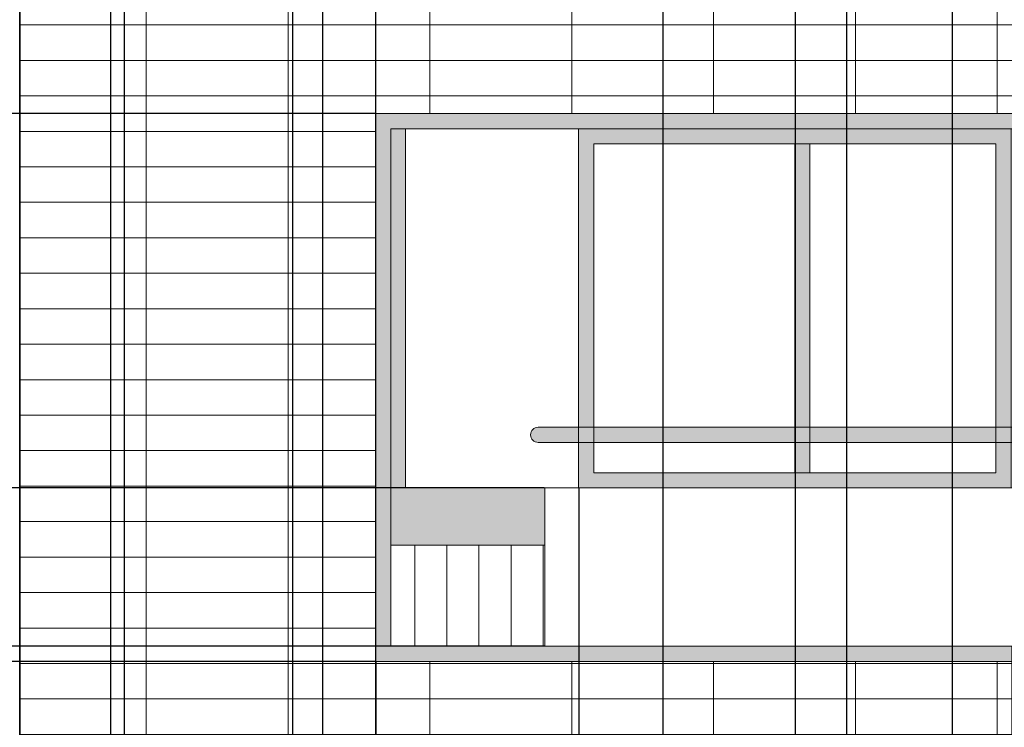
# Model space of a CAD drawing. Units: inches. Extents: x 241 to 943, y 109 to 1396.
# Tile 10 of 34: x 377 to 507, y 620 to 713. Entities that reach past the tile are written whole.
import ezdxf

# ---------------------------------------------------------------- set-up
doc = ezdxf.new("R2010")
doc.units = ezdxf.units.IN
doc.header["$MEASUREMENT"] = 0
for name, color, linetype, lineweight in [('A-ANNO-DIMS', 2, 'Continuous', 18), ('A-ELEV', 7, 'Continuous', 25), ('A-ELEV-SHAD', 9, 'Continuous', 13), ('A-GLAZ', 4, 'Continuous', 18), ('A-GLAZ-PATT', 18, 'Continuous', 13), ('A-WALL-PATT', 8, 'Continuous', 13)]:
    doc.layers.add(name, color=color, linetype=linetype, lineweight=lineweight)
doc.styles.get("Standard").update_dxf_attribs({"font": 'arial.ttf'})
doc.dimstyles.get("Standard").update_dxf_attribs({"dimtxt": 1.4375, "dimasz": 0.18, "dimexe": 0.18, "dimexo": 0.0625, "dimgap": 0.09, "dimtad": 0, "dimtih": 1, "dimtoh": 1, "dimdec": 4, "dimzin": 0, "dimdsep": 46, "dimlunit": 4, "dimtxsty": 'Standard', "dimcen": 0.09, "dimadec": 0, "dimazin": 0, "dimtfac": 1, "dimtdec": 4, "dimtofl": 0, "dimtmove": 0, "dimatfit": 3, "dimfxl": 1, "dimtolj": 1, "dimtzin": 0, "dimarcsym": 0})

# ---------------------------------------------------------------- blocks, each defined once
blk = doc.blocks.new('*D7')
at = {"layer": 'A-ANNO-DIMS', "color": 0, "lineweight": -2, "transparency": 16777216}
for p, q in [((508.24, 1336.12), (244.31, 1336.12)), ((244.49, 1335.94), (244.49, 753.25)), ((244.49, 168.92), (244.49, 751.6)), ((303.17, 168.74), (244.31, 168.74))]:
    blk.add_line(p, q, dxfattribs=at)
at = {"layer": 'A-ANNO-DIMS', "color": 0, "transparency": 16777216}
for points in [[(244.46, 1335.94), (244.52, 1335.94), (244.49, 1336.12)], [(244.46, 168.92), (244.52, 168.92), (244.49, 168.74)]]:
    blk.add_solid(points, dxfattribs=at)
at = {"layer": 'Defpoints', "color": 0, "transparency": 16777216}
for p in [(244.49, 1336.12), (508.31, 1336.12), (303.24, 168.74)]:
    blk.add_point(p, dxfattribs=at)
at = {"layer": 'A-ANNO-DIMS', "color": 0, "transparency": 16777216, "insert": (244.49, 752.43), "char_height": 1.438, "attachment_point": 5}
blk.add_mtext('\\A1;1167.4', dxfattribs=at)
blk = doc.blocks.new('*D8')
at = {"layer": 'A-ANNO-DIMS', "color": 0, "lineweight": -2, "transparency": 16777216}
for p, q in [((377.04, 396.94), (377.04, 1395.05)), ((377.22, 1394.87), (380.96, 1394.87)), ((390.71, 1394.87), (386.97, 1394.87)), ((390.89, 384.24), (390.89, 1395.05))]:
    blk.add_line(p, q, dxfattribs=at)
at = {"layer": 'A-ANNO-DIMS', "color": 0, "transparency": 16777216}
for points in [[(377.22, 1394.9), (377.22, 1394.84), (377.04, 1394.87)], [(390.71, 1394.9), (390.71, 1394.84), (390.89, 1394.87)]]:
    blk.add_solid(points, dxfattribs=at)
at = {"layer": 'Defpoints', "color": 0, "transparency": 16777216}
for p in [(390.89, 1394.87), (377.04, 396.88), (390.89, 384.18)]:
    blk.add_point(p, dxfattribs=at)
at = {"layer": 'A-ANNO-DIMS', "color": 0, "transparency": 16777216, "insert": (383.97, 1394.87), "char_height": 1.438, "attachment_point": 5}
blk.add_mtext('\\A1;13.856', dxfattribs=at)
blk = doc.blocks.new('*D9')
at = {"layer": 'A-ANNO-DIMS', "color": 0, "lineweight": -2, "transparency": 16777216}
for p, q in [((390.89, 384.24), (390.89, 1395.05)), ((391.07, 1394.87), (424.13, 1394.87)), ((461.93, 1394.87), (428.87, 1394.87)), ((462.11, 384.24), (462.11, 1395.05))]:
    blk.add_line(p, q, dxfattribs=at)
at = {"layer": 'A-ANNO-DIMS', "color": 0, "transparency": 16777216}
for points in [[(391.07, 1394.9), (391.07, 1394.84), (390.89, 1394.87)], [(461.93, 1394.9), (461.93, 1394.84), (462.11, 1394.87)]]:
    blk.add_solid(points, dxfattribs=at)
at = {"layer": 'Defpoints', "color": 0, "transparency": 16777216}
for p in [(462.11, 1394.87), (390.89, 384.18), (462.11, 384.18)]:
    blk.add_point(p, dxfattribs=at)
at = {"layer": 'A-ANNO-DIMS', "color": 0, "transparency": 16777216, "insert": (426.5, 1394.87), "char_height": 1.438, "attachment_point": 5}
blk.add_mtext('\\A1;71.21', dxfattribs=at)
blk = doc.blocks.new('*D10')
at = {"layer": 'A-ANNO-DIMS', "color": 0, "lineweight": -2, "transparency": 16777216}
for p, q in [((462.11, 384.24), (462.11, 1395.05)), ((462.29, 1394.87), (468.4, 1394.87)), ((479.42, 1394.87), (473.3, 1394.87)), ((479.6, 384.24), (479.6, 1395.05))]:
    blk.add_line(p, q, dxfattribs=at)
at = {"layer": 'A-ANNO-DIMS', "color": 0, "transparency": 16777216}
for points in [[(462.29, 1394.9), (462.29, 1394.84), (462.11, 1394.87)], [(479.42, 1394.9), (479.42, 1394.84), (479.6, 1394.87)]]:
    blk.add_solid(points, dxfattribs=at)
at = {"layer": 'Defpoints', "color": 0, "transparency": 16777216}
for p in [(479.6, 1394.87), (462.11, 384.18), (479.6, 384.18)]:
    blk.add_point(p, dxfattribs=at)
at = {"layer": 'A-ANNO-DIMS', "color": 0, "transparency": 16777216, "insert": (470.85, 1394.87), "char_height": 1.438, "attachment_point": 5}
blk.add_mtext('\\A1;17.49', dxfattribs=at)
blk = doc.blocks.new('*D11')
at = {"layer": 'A-ANNO-DIMS', "color": 0, "lineweight": -2, "transparency": 16777216}
for p, q in [((500.33, 384.24), (500.33, 1395.05)), ((500.51, 1394.87), (513.31, 1394.87)), ((530.05, 1394.87), (517.25, 1394.87)), ((530.23, 384.24), (530.23, 1395.05))]:
    blk.add_line(p, q, dxfattribs=at)
at = {"layer": 'A-ANNO-DIMS', "color": 0, "transparency": 16777216}
for points in [[(500.51, 1394.9), (500.51, 1394.84), (500.33, 1394.87)], [(530.05, 1394.9), (530.05, 1394.84), (530.23, 1394.87)]]:
    blk.add_solid(points, dxfattribs=at)
at = {"layer": 'Defpoints', "color": 0, "transparency": 16777216}
for p in [(530.23, 1394.87), (500.33, 384.18), (530.23, 384.18)]:
    blk.add_point(p, dxfattribs=at)
at = {"layer": 'A-ANNO-DIMS', "color": 0, "transparency": 16777216, "insert": (515.28, 1394.87), "char_height": 1.438, "attachment_point": 5}
blk.add_mtext('\\A1;29.9', dxfattribs=at)
blk = doc.blocks.new('*D33')
at = {"layer": 'A-ANNO-DIMS', "color": 0, "lineweight": -2, "transparency": 16777216}
for p, q in [((424.05, 628.4), (244.31, 628.4)), ((244.49, 628.22), (244.49, 599.44)), ((244.49, 569.01), (244.49, 597.79)), ((424.05, 568.83), (244.31, 568.83))]:
    blk.add_line(p, q, dxfattribs=at)
at = {"layer": 'A-ANNO-DIMS', "color": 0, "transparency": 16777216}
for points in [[(244.46, 628.22), (244.52, 628.22), (244.49, 628.4)], [(244.46, 569.01), (244.52, 569.01), (244.49, 568.83)]]:
    blk.add_solid(points, dxfattribs=at)
at = {"layer": 'Defpoints', "color": 0, "transparency": 16777216}
for p in [(244.49, 628.4), (424.11, 628.4), (424.11, 568.83)]:
    blk.add_point(p, dxfattribs=at)
at = {"layer": 'A-ANNO-DIMS', "color": 0, "transparency": 16777216, "insert": (244.49, 598.62), "char_height": 1.438, "attachment_point": 5}
blk.add_mtext('\\A1;59.57', dxfattribs=at)
blk = doc.blocks.new('*D34')
at = {"layer": 'A-ANNO-DIMS', "color": 0, "lineweight": -2, "transparency": 16777216}
for p, q in [((424.05, 700.79), (244.31, 700.79)), ((244.49, 700.61), (244.49, 665.42)), ((244.49, 628.58), (244.49, 663.77)), ((424.05, 628.4), (244.31, 628.4))]:
    blk.add_line(p, q, dxfattribs=at)
at = {"layer": 'A-ANNO-DIMS', "color": 0, "transparency": 16777216}
for points in [[(244.46, 700.61), (244.52, 700.61), (244.49, 700.79)], [(244.46, 628.58), (244.52, 628.58), (244.49, 628.4)]]:
    blk.add_solid(points, dxfattribs=at)
at = {"layer": 'Defpoints', "color": 0, "transparency": 16777216}
for p in [(244.49, 700.79), (424.11, 700.79), (424.11, 628.4)]:
    blk.add_point(p, dxfattribs=at)
at = {"layer": 'A-ANNO-DIMS', "color": 0, "transparency": 16777216, "insert": (244.49, 664.6), "char_height": 1.438, "attachment_point": 5}
blk.add_mtext('\\A1;72.39', dxfattribs=at)
blk = doc.blocks.new('*D61')
at = {"layer": 'A-ANNO-DIMS', "color": 0, "lineweight": -2, "transparency": 16777216}
for p, q in [((377.04, 400.89), (377.04, 1395.05)), ((377.22, 1394.87), (398.03, 1394.87)), ((423.93, 1394.87), (403.12, 1394.87)), ((424.11, 568.89), (424.11, 1395.05))]:
    blk.add_line(p, q, dxfattribs=at)
at = {"layer": 'A-ANNO-DIMS', "color": 0, "transparency": 16777216}
for points in [[(377.22, 1394.9), (377.22, 1394.84), (377.04, 1394.87)], [(423.93, 1394.9), (423.93, 1394.84), (424.11, 1394.87)]]:
    blk.add_solid(points, dxfattribs=at)
at = {"layer": 'Defpoints', "color": 0, "transparency": 16777216}
for p in [(424.11, 1394.87), (424.11, 568.83), (377.04, 400.83)]:
    blk.add_point(p, dxfattribs=at)
at = {"layer": 'A-ANNO-DIMS', "color": 0, "transparency": 16777216, "insert": (400.57, 1394.87), "char_height": 1.438, "attachment_point": 5}
blk.add_mtext('\\A1;47.07', dxfattribs=at)
blk = doc.blocks.new('*D62')
at = {"layer": 'A-ANNO-DIMS', "color": 0, "lineweight": -2, "transparency": 16777216}
for p, q in [((424.11, 568.89), (424.11, 1395.05)), ((424.29, 1394.87), (492.35, 1394.87)), ((565.02, 1394.87), (496.96, 1394.87)), ((565.2, 568.89), (565.2, 1395.05))]:
    blk.add_line(p, q, dxfattribs=at)
at = {"layer": 'A-ANNO-DIMS', "color": 0, "transparency": 16777216}
for points in [[(424.29, 1394.9), (424.29, 1394.84), (424.11, 1394.87)], [(565.02, 1394.9), (565.02, 1394.84), (565.2, 1394.87)]]:
    blk.add_solid(points, dxfattribs=at)
at = {"layer": 'Defpoints', "color": 0, "transparency": 16777216}
for p in [(565.2, 1394.87), (424.11, 568.83), (565.2, 568.83)]:
    blk.add_point(p, dxfattribs=at)
at = {"layer": 'A-ANNO-DIMS', "color": 0, "transparency": 16777216, "insert": (494.66, 1394.87), "char_height": 1.438, "attachment_point": 5}
blk.add_mtext('\\A1;141.1', dxfattribs=at)
blk = doc.blocks.new('*D65')
at = {"layer": 'A-ANNO-DIMS', "color": 0, "lineweight": -2, "transparency": 16777216}
for p, q in [((424.11, 700.85), (424.11, 1395.05)), ((424.29, 1394.87), (505.52, 1394.87)), ((592.77, 1394.87), (511.54, 1394.87)), ((592.95, 700.85), (592.95, 1395.05))]:
    blk.add_line(p, q, dxfattribs=at)
at = {"layer": 'A-ANNO-DIMS', "color": 0, "transparency": 16777216}
for points in [[(424.29, 1394.9), (424.29, 1394.84), (424.11, 1394.87)], [(592.77, 1394.9), (592.77, 1394.84), (592.95, 1394.87)]]:
    blk.add_solid(points, dxfattribs=at)
at = {"layer": 'Defpoints', "color": 0, "transparency": 16777216}
for p in [(592.95, 1394.87), (424.11, 700.79), (592.95, 700.79)]:
    blk.add_point(p, dxfattribs=at)
at = {"layer": 'A-ANNO-DIMS', "color": 0, "transparency": 16777216, "insert": (508.53, 1394.87), "char_height": 1.438, "attachment_point": 5}
blk.add_mtext('\\A1;168.85', dxfattribs=at)
blk = doc.blocks.new('*D79')
at = {"layer": 'A-ANNO-DIMS', "color": 0, "lineweight": -2, "transparency": 16777216}
for p, q in [((479.6, 384.24), (479.6, 1395.05)), ((479.78, 1394.87), (486.88, 1394.87)), ((500.15, 1394.87), (493.05, 1394.87)), ((500.33, 384.24), (500.33, 1395.05))]:
    blk.add_line(p, q, dxfattribs=at)
at = {"layer": 'A-ANNO-DIMS', "color": 0, "transparency": 16777216}
for points in [[(479.78, 1394.9), (479.78, 1394.84), (479.6, 1394.87)], [(500.15, 1394.9), (500.15, 1394.84), (500.33, 1394.87)]]:
    blk.add_solid(points, dxfattribs=at)
at = {"layer": 'Defpoints', "color": 0, "transparency": 16777216}
for p in [(500.33, 1394.87), (479.6, 384.18), (500.33, 384.18)]:
    blk.add_point(p, dxfattribs=at)
at = {"layer": 'A-ANNO-DIMS', "color": 0, "transparency": 16777216, "insert": (489.96, 1394.87), "char_height": 1.438, "attachment_point": 5}
blk.add_mtext('\\A1;20.736', dxfattribs=at)
blk = doc.blocks.new('*D91')
at = {"layer": 'A-ANNO-DIMS', "color": 0, "lineweight": -2, "transparency": 16777216}
for p, q in [((377.04, 1070.79), (377.04, 109.81)), ((389.04, 1070.79), (389.04, 109.81)), ((377.22, 109.99), (380.04, 109.99)), ((388.86, 109.99), (386.04, 109.99))]:
    blk.add_line(p, q, dxfattribs=at)
at = {"layer": 'A-ANNO-DIMS', "color": 0, "transparency": 16777216}
for points in [[(377.22, 110.02), (377.22, 109.96), (377.04, 109.99)], [(388.86, 110.02), (388.86, 109.96), (389.04, 109.99)]]:
    blk.add_solid(points, dxfattribs=at)
at = {"layer": 'Defpoints', "color": 0, "transparency": 16777216}
for p in [(377.04, 1070.85), (389.04, 1070.85), (389.04, 109.99)]:
    blk.add_point(p, dxfattribs=at)
at = {"layer": 'A-ANNO-DIMS', "color": 0, "transparency": 16777216, "insert": (383.04, 109.99), "char_height": 1.438, "attachment_point": 5}
blk.add_mtext('\\A1;12.004', dxfattribs=at)
blk = doc.blocks.new('*D99')
at = {"layer": 'A-ANNO-DIMS', "color": 0, "lineweight": -2, "transparency": 16777216}
for p, q in [((417.09, 181.71), (417.09, 1395.05)), ((417.27, 1394.87), (539.16, 1394.87)), ((667.21, 1394.87), (545.33, 1394.87)), ((667.39, 214.58), (667.39, 1395.05))]:
    blk.add_line(p, q, dxfattribs=at)
at = {"layer": 'A-ANNO-DIMS', "color": 0, "transparency": 16777216}
for points in [[(417.27, 1394.9), (417.27, 1394.84), (417.09, 1394.87)], [(667.21, 1394.9), (667.21, 1394.84), (667.39, 1394.87)]]:
    blk.add_solid(points, dxfattribs=at)
at = {"layer": 'Defpoints', "color": 0, "transparency": 16777216}
for p in [(667.39, 1394.87), (667.39, 214.52), (417.09, 181.65)]:
    blk.add_point(p, dxfattribs=at)
at = {"layer": 'A-ANNO-DIMS', "color": 0, "transparency": 16777216, "insert": (542.24, 1394.87), "char_height": 1.438, "attachment_point": 5}
blk.add_mtext('\\A1;250.30', dxfattribs=at)
blk = doc.blocks.new('*D126')
at = {"layer": 'A-ANNO-DIMS', "color": 0, "lineweight": -2, "transparency": 16777216}
for p, q in [((450.93, 651.27), (450.93, 109.81)), ((424.11, 628.34), (424.11, 109.81)), ((424.29, 109.99), (434.43, 109.99)), ((450.75, 109.99), (440.6, 109.99))]:
    blk.add_line(p, q, dxfattribs=at)
at = {"layer": 'A-ANNO-DIMS', "color": 0, "transparency": 16777216}
for points in [[(424.29, 110.02), (424.29, 109.96), (424.11, 109.99)], [(450.75, 110.02), (450.75, 109.96), (450.93, 109.99)]]:
    blk.add_solid(points, dxfattribs=at)
at = {"layer": 'Defpoints', "color": 0, "transparency": 16777216}
for p in [(450.93, 651.34), (424.11, 628.4), (450.93, 109.99)]:
    blk.add_point(p, dxfattribs=at)
at = {"layer": 'A-ANNO-DIMS', "color": 0, "transparency": 16777216, "insert": (437.52, 109.99), "char_height": 1.438, "attachment_point": 5}
blk.add_mtext('\\A1;26.817', dxfattribs=at)
blk = doc.blocks.new('*D127')
at = {"layer": 'A-ANNO-DIMS', "color": 0, "lineweight": -2, "transparency": 16777216}
for p, q in [((450.93, 651.27), (450.93, 109.81)), ((508.19, 630.34), (508.19, 109.81)), ((451.11, 109.99), (477.04, 109.99)), ((508.01, 109.99), (482.07, 109.99))]:
    blk.add_line(p, q, dxfattribs=at)
at = {"layer": 'A-ANNO-DIMS', "color": 0, "transparency": 16777216}
for points in [[(451.11, 110.02), (451.11, 109.96), (450.93, 109.99)], [(508.01, 110.02), (508.01, 109.96), (508.19, 109.99)]]:
    blk.add_solid(points, dxfattribs=at)
at = {"layer": 'Defpoints', "color": 0, "transparency": 16777216}
for p in [(450.93, 651.34), (508.19, 630.4), (508.19, 109.99)]:
    blk.add_point(p, dxfattribs=at)
at = {"layer": 'A-ANNO-DIMS', "color": 0, "transparency": 16777216, "insert": (479.56, 109.99), "char_height": 1.438, "attachment_point": 5}
blk.add_mtext('\\A1;57.26', dxfattribs=at)
blk = doc.blocks.new('*D131')
at = {"layer": 'A-ANNO-DIMS', "color": 0, "lineweight": -2, "transparency": 16777216}
for p, q in [((446.37, 651.34), (244.31, 651.34)), ((244.49, 651.16), (244.49, 641.69)), ((244.49, 630.58), (244.49, 640.04)), ((446.37, 630.4), (244.31, 630.4))]:
    blk.add_line(p, q, dxfattribs=at)
at = {"layer": 'A-ANNO-DIMS', "color": 0, "transparency": 16777216}
for points in [[(244.46, 651.16), (244.52, 651.16), (244.49, 651.34)], [(244.46, 630.58), (244.52, 630.58), (244.49, 630.4)]]:
    blk.add_solid(points, dxfattribs=at)
at = {"layer": 'Defpoints', "color": 0, "transparency": 16777216}
for p in [(244.49, 651.34), (446.43, 651.34), (446.43, 630.4)]:
    blk.add_point(p, dxfattribs=at)
at = {"layer": 'A-ANNO-DIMS', "color": 0, "transparency": 16777216, "insert": (244.49, 640.87), "char_height": 1.438, "attachment_point": 5}
blk.add_mtext('\\A1;20.936', dxfattribs=at)
blk = doc.blocks.new('*D147')
at = {"layer": 'A-ANNO-DIMS', "color": 0, "lineweight": -2, "transparency": 16777216}
for p, q in [((389.04, 734.79), (389.04, 109.81)), ((413.12, 734.79), (413.12, 109.81)), ((389.22, 109.99), (398, 109.99)), ((412.94, 109.99), (404.17, 109.99))]:
    blk.add_line(p, q, dxfattribs=at)
at = {"layer": 'A-ANNO-DIMS', "color": 0, "transparency": 16777216}
for points in [[(389.22, 110.02), (389.22, 109.96), (389.04, 109.99)], [(412.94, 110.02), (412.94, 109.96), (413.12, 109.99)]]:
    blk.add_solid(points, dxfattribs=at)
at = {"layer": 'Defpoints', "color": 0, "transparency": 16777216}
for p in [(389.04, 734.85), (413.12, 734.85), (413.12, 109.99)]:
    blk.add_point(p, dxfattribs=at)
at = {"layer": 'A-ANNO-DIMS', "color": 0, "transparency": 16777216, "insert": (401.08, 109.99), "char_height": 1.438, "attachment_point": 5}
blk.add_mtext('\\A1;24.076', dxfattribs=at)
blk = doc.blocks.new('*D148')
at = {"layer": 'A-ANNO-DIMS', "color": 0, "lineweight": -2, "transparency": 16777216}
for p, q in [((413.12, 734.79), (413.12, 109.81)), ((486.34, 734.79), (486.34, 109.81)), ((413.3, 109.99), (447.23, 109.99)), ((486.16, 109.99), (452.23, 109.99))]:
    blk.add_line(p, q, dxfattribs=at)
at = {"layer": 'A-ANNO-DIMS', "color": 0, "transparency": 16777216}
for points in [[(413.3, 110.02), (413.3, 109.96), (413.12, 109.99)], [(486.16, 110.02), (486.16, 109.96), (486.34, 109.99)]]:
    blk.add_solid(points, dxfattribs=at)
at = {"layer": 'Defpoints', "color": 0, "transparency": 16777216}
for p in [(413.12, 734.85), (486.34, 734.85), (486.34, 109.99)]:
    blk.add_point(p, dxfattribs=at)
at = {"layer": 'A-ANNO-DIMS', "color": 0, "transparency": 16777216, "insert": (449.73, 109.99), "char_height": 1.438, "attachment_point": 5}
blk.add_mtext('\\A1;73.22', dxfattribs=at)

msp = doc.modelspace()

# ---------------------------------------------------------------- hatches: boundary and pattern name
at = {"layer": 'A-ELEV-SHAD'}
h = msp.add_hatch(color=256, dxfattribs=at)
h.dxf.hatch_style = 1
h.paths.add_polyline_path([(537.4269, 698.7912), (534.1778, 698.7912), (534.1778, 659.3434), (537.4269, 659.3434)])
h.paths.add_polyline_path([(508.0803, 698.7912), (450.9259, 698.7912), (450.9259, 659.3434), (452.9259, 659.3434), (452.9259, 696.7912), (506.0803, 696.7912), (506.0803, 659.3434), (508.0803, 659.3434)])
h.paths.add_polyline_path([(481.5031, 696.7912), (479.5031, 696.7912), (479.5031, 659.3434), (481.5031, 659.3434)], flags=17)
h.paths.add_polyline_path([(481.5031, 657.3434), (479.5031, 657.3434), (479.5031, 653.3371), (481.5031, 653.3371)], flags=17)
h.paths.add_polyline_path([(508.0803, 657.3434), (506.0803, 657.3434), (506.0803, 653.3371), (452.9259, 653.3371), (452.9259, 657.3434), (450.9259, 657.3434), (450.9259, 651.3371), (508.0803, 651.3371)])
h.paths.add_polyline_path([(428.1173, 839.5382), (426.1173, 839.5382), (426.1173, 786.9154), (428.1173, 786.9154)], flags=17)
h.paths.add_polyline_path([(470.8692, 839.5382), (468.8692, 839.5382), (468.8692, 786.9154), (470.8692, 786.9154)], flags=17)
h.paths.add_polyline_path([(508.3064, 841.5382), (396.3125, 841.5382), (396.3125, 782.5808), (398.3125, 782.5808), (398.3125, 839.5382), (506.3064, 839.5382), (506.3064, 782.5808), (508.3064, 782.5808)])
h.paths.add_polyline_path([(398.3125, 780.5808), (396.3125, 780.5808), (396.3125, 773.4916), (398.3125, 773.4916)])
h.paths.add_polyline_path([(508.3064, 780.5808), (506.3064, 780.5808), (506.3064, 773.4916), (508.3064, 773.4916)])
h.paths.add_polyline_path([(715.6236, 841.5382), (678.2674, 841.5382), (678.2674, 734.8538), (715.6236, 734.8538)])
h.paths.add_polyline_path([(680.2674, 839.5382), (682.4526, 839.5382), (713.6236, 839.5382), (713.6236, 736.9235), (690.2047, 736.9235), (680.2674, 736.9235)], flags=16)
h.paths.add_polyline_path([(792.691, 841.5382), (747.7579, 841.5382), (747.7579, 734.8538), (754.5373, 734.8538), (754.5373, 736.9235), (754.5373, 839.5382), (756.7224, 839.5382), (787.8934, 839.5382), (787.8934, 765.9585), (792.691, 765.9585)])
h.paths.add_polyline_path([(659.2925, 1009.5382), (657.2925, 1009.5382), (657.2925, 902.8538), (659.2925, 902.8538)])
h.paths.add_polyline_path([(751.5078, 976.6275), (712.5839, 976.6275), (712.5839, 974.6275), (751.5078, 974.6275)])
h.paths.add_polyline_path([(470.8692, 1007.5382), (468.8692, 1007.5382), (468.8692, 954.9154), (470.8692, 954.9154)], flags=17)
h.paths.add_polyline_path([(508.3064, 1009.5382), (396.3125, 1009.5382), (396.3125, 950.5808), (398.3125, 950.5808), (398.3125, 1007.5382), (506.3064, 1007.5382), (506.3064, 950.5808), (508.3064, 950.5808)])
h.paths.add_polyline_path([(428.1173, 1007.5382), (426.1173, 1007.5382), (426.1173, 954.9154), (428.1173, 954.9154)], flags=17)
h.paths.add_polyline_path([(398.3125, 948.5808), (396.3125, 948.5808), (396.3125, 941.4916), (398.3125, 941.4916)])
h.paths.add_polyline_path([(508.3064, 948.5808), (506.3064, 948.5808), (506.3064, 941.4916), (508.3064, 941.4916)])
h.paths.add_polyline_path([(428.1173, 1175.5382), (426.1173, 1175.5382), (426.1173, 1122.9154), (428.1173, 1122.9154)], flags=17)
h.paths.add_polyline_path([(508.3064, 1177.5382), (396.3125, 1177.5382), (396.3125, 1118.5808), (398.3125, 1118.5808), (398.3125, 1175.5382), (506.3064, 1175.5382), (506.3064, 1118.5808), (506.8039, 1118.5808, -1), (506.8039, 1116.5808), (506.3064, 1116.5808), (506.3064, 1109.4916), (508.3064, 1109.4916)])
h.paths.add_polyline_path([(470.8692, 1175.5382), (468.8692, 1175.5382), (468.8692, 1122.9154), (470.8692, 1122.9154)], flags=17)
h.paths.add_polyline_path([(398.3125, 1116.5808), (396.3125, 1116.5808), (396.3125, 1109.4916), (398.3125, 1109.4916)], flags=17)
h.paths.add_polyline_path([(724.819, 1177.7336), (533.952, 1177.7336), (533.952, 1108.1686), (724.819, 1108.1686)])
h.paths.add_polyline_path([(535.952, 1175.7336), (722.819, 1175.7336), (722.819, 1110.1686), (535.952, 1110.1686)], flags=0)
h.paths.add_polyline_path([(622.521, 1136.0739), (643.4534, 1136.0739), (643.4534, 1134.0739), (622.521, 1134.0739)], flags=0)
h.paths.add_polyline_path([(722.819, 1175.7336), (535.952, 1175.7336), (535.952, 1110.1686), (722.819, 1110.1686)], flags=16)
h.paths.add_polyline_path([(565.947, 1151.5772), (535.952, 1151.5772), (535.952, 1149.5772), (565.947, 1149.5772)], flags=0)
h = msp.add_hatch(color=256, dxfattribs=at)
h.dxf.hatch_style = 1
h.paths.add_polyline_path([(759.6248, 762.5799), (792.691, 762.5799), (792.691, 765.9585), (754.5373, 765.9585), (754.5373, 736.9235), (754.5373, 734.8538), (759.6248, 734.8538), (759.6248, 736.9235)])
h.paths.add_polyline_path([(446.4348, 651.3371), (428.0291, 651.3371), (428.0291, 698.7912), (426.1086, 698.7912), (426.1086, 643.7483), (446.4348, 643.7483)])
h = msp.add_hatch(color=256, dxfattribs=at)
h.dxf.hatch_style = 1
h.paths.add_polyline_path([(537.4269, 566.8295), (534.1778, 566.8295), (534.1778, 527.3816), (537.4269, 527.3816)])
h.paths.add_polyline_path([(508.0803, 566.8295), (450.9259, 566.8295), (450.9259, 527.3816), (452.9259, 527.3816), (452.9259, 564.8295), (506.0803, 564.8295), (506.0803, 527.3816), (508.0803, 527.3816)])
h.paths.add_polyline_path([(481.5031, 564.8295), (479.5031, 564.8295), (479.5031, 527.3816), (481.5031, 527.3816)], flags=17)
h.paths.add_polyline_path([(481.5031, 525.3816), (479.5031, 525.3816), (479.5031, 521.3754), (481.5031, 521.3754)], flags=17)
h.paths.add_polyline_path([(508.0803, 525.3816), (506.0803, 525.3816), (506.0803, 521.3754), (452.9259, 521.3754), (452.9259, 525.3816), (450.9259, 525.3816), (450.9259, 519.3754), (508.0803, 519.3754)])
h.paths.add_polyline_path([(537.4269, 525.3816), (534.1778, 525.3816), (534.1778, 508.9074), (537.4269, 508.9074)])
h.paths.add_polyline_path([(749.6328, 702.7912), (617.7594, 702.7912), (617.7594, 700.7912), (747.6328, 700.7912), (747.6328, 628.4013), (617.7594, 628.4013), (617.7594, 626.4013), (749.6328, 626.4013)])
h.paths.add_polyline_path([(652.0129, 700.7912), (650.0129, 700.7912), (650.0129, 628.4013), (652.0129, 628.4013)], flags=17)
h.paths.add_polyline_path([(678.8698, 700.7912), (676.8698, 700.7912), (676.8698, 628.4013), (678.8698, 628.4013)], flags=17)
h.paths.add_polyline_path([(712.0171, 700.7912), (710.0171, 700.7912), (710.0171, 628.4013), (712.0171, 628.4013)], flags=17)
h.paths.add_polyline_path([(710.0171, 675.7856), (678.8698, 675.7856), (678.8698, 673.7856), (710.0171, 673.7856)], flags=17)
h.paths.add_polyline_path([(537.4269, 698.7912), (534.1778, 698.7912), (534.1778, 659.3434), (537.4269, 659.3434)], flags=0)
h.paths.add_polyline_path([(592.9542, 700.7912), (424.1086, 700.7912), (424.1086, 628.4013), (592.9542, 628.4013)])
h.paths.add_polyline_path([(590.8792, 698.7912), (590.8792, 630.4013), (426.1086, 630.4013), (426.1086, 698.7912)], flags=16)
h.paths.add_polyline_path([(563.2023, 698.7912), (563.2023, 659.3434), (563.9297, 659.3434), (563.9297, 651.3371), (508.1906, 651.3371), (508.0803, 651.3371), (450.9259, 651.3371), (428.0291, 651.3371), (428.0291, 698.7912), (451.9767, 698.7912), (508.0803, 698.7912), (537.4269, 698.7912)], flags=0)
h.paths.add_polyline_path([(506.0803, 696.7912), (506.0803, 653.3371), (452.9259, 653.3371), (452.9259, 657.3434), (445.5808, 657.3434, -1), (445.5808, 659.3434), (452.9259, 659.3434), (452.9259, 696.7912)], flags=0)
h.paths.add_polyline_path([(563.9297, 698.7912), (563.2023, 698.7912), (563.2023, 659.3434), (563.9297, 659.3434)], flags=0)
at = {"layer": 'A-GLAZ-PATT'}
h = msp.add_hatch(dxfattribs=at)
h.set_pattern_fill('ANSI31', color=256, scale=34, angle=45)
h.paths.add_polyline_path([(486.3418, 786.9154), (413.1187, 786.9154), (413.1187, 761.2284), (486.3418, 761.2284)])
h.paths.add_polyline_path([(486.3418, 954.9154), (413.1187, 954.9154), (413.1187, 929.2284), (486.3418, 929.2284)])
h.paths.add_polyline_path([(462.1074, 289.6933), (390.895, 289.6933), (390.895, 277.4626), (390.895, 274.3507), (462.1074, 274.3507), (462.1074, 277.4626)])
h.paths.add_polyline_path([(500.3323, 289.6933), (479.596, 289.6933), (479.596, 274.3507), (500.3323, 274.3507)])
h.paths.add_polyline_path([(450.9259, 566.8295), (426.1086, 566.8295), (426.1086, 498.4395), (446.4348, 498.4395), (446.4348, 519.3754), (450.9259, 519.3754), (450.9259, 525.3816), (445.5808, 525.3816, -1), (445.5808, 527.3816), (450.9259, 527.3816)])
h.paths.add_polyline_path([(563.2023, 508.9074), (534.1778, 508.9074), (508.1906, 508.9074), (508.1906, 498.4395), (563.2023, 498.4395)])
h.paths.add_polyline_path([(747.6328, 700.7912), (712.0171, 700.7912), (712.0171, 628.4013), (747.6328, 628.4013)])
h.paths.add_polyline_path([(446.4348, 643.7483), (426.1086, 643.7483), (426.1086, 630.4013), (446.4348, 630.4013)])
h.paths.add_polyline_path([(564.8076, 841.5382), (553.5166, 841.5382), (508.3064, 841.5382), (508.3064, 782.5808), (564.8076, 782.5808)])
h.paths.add_polyline_path([(564.8076, 780.5808), (508.3064, 780.5808), (508.3064, 773.4916), (564.8076, 773.4916)])
h.paths.add_polyline_path([(792.691, 762.5799), (759.6248, 762.5799), (759.6248, 736.9235), (759.6248, 734.8538), (792.691, 734.8538)])
h.paths.add_polyline_path([(564.8076, 1009.5382), (553.5166, 1009.5382), (508.3064, 1009.5382), (508.3064, 950.5808), (562.3033, 950.5808, -1), (562.3033, 948.5808), (508.3064, 948.5808), (508.3064, 941.4916), (564.8076, 941.4916)])
h.paths.add_polyline_path([(486.3418, 1122.9154), (413.1187, 1122.9154), (413.1187, 1097.2284), (486.3418, 1097.2284)])
h = msp.add_hatch(color=256, dxfattribs=at)
h.dxf.hatch_style = 1
h.paths.add_polyline_path([(396.3125, 1118.5808), (390.5597, 1118.5808), (388.0428, 1118.5808, 1), (388.0428, 1116.5808), (390.5597, 1116.5808), (396.3125, 1116.5808)])
h.paths.add_polyline_path([(398.3125, 1118.5808), (396.3125, 1118.5808), (396.3125, 1116.5808), (398.3125, 1116.5808)])
h.paths.add_polyline_path([(413.1187, 1118.5808), (398.3125, 1118.5808), (398.3125, 1116.5808), (413.1187, 1116.5808)])
h.paths.add_polyline_path([(506.3064, 1118.5808), (486.3418, 1118.5808), (486.3418, 1116.5808), (506.3064, 1116.5808)])
h.paths.add_polyline_path([(506.8039, 1118.5808), (506.3064, 1118.5808), (506.3064, 1116.5808), (506.8039, 1116.5808, 1)])
h.paths.add_polyline_path([(396.3125, 950.5808), (390.5597, 950.5808), (388.0428, 950.5808, 1), (388.0428, 948.5808), (390.5597, 948.5808), (396.3125, 948.5808)])
h.paths.add_polyline_path([(398.3125, 950.5808), (396.3125, 950.5808), (396.3125, 948.5808), (398.3125, 948.5808)])
h.paths.add_polyline_path([(413.1187, 950.5808), (398.3125, 950.5808), (398.3125, 948.5808), (413.1187, 948.5808)])
h.paths.add_polyline_path([(506.3064, 950.5808), (486.3418, 950.5808), (486.3418, 948.5808), (506.3064, 948.5808)])
h.paths.add_polyline_path([(508.3064, 950.5808), (506.3064, 950.5808), (506.3064, 948.5808), (508.3064, 948.5808)])
h.paths.add_polyline_path([(562.3033, 950.5808), (508.3064, 950.5808), (508.3064, 948.5808), (562.3033, 948.5808, 1)])
h.paths.add_polyline_path([(396.3125, 782.5808), (390.5597, 782.5808), (388.0428, 782.5808, 1), (388.0428, 780.5808), (390.5597, 780.5808), (396.3125, 780.5808)])
h.paths.add_polyline_path([(398.3125, 782.5808), (396.3125, 782.5808), (396.3125, 780.5808), (398.3125, 780.5808)])
h.paths.add_polyline_path([(413.1187, 782.5808), (398.3125, 782.5808), (398.3125, 780.5808), (413.1187, 780.5808)])
h.paths.add_polyline_path([(506.3064, 782.5808), (486.3418, 782.5808), (486.3418, 780.5808), (506.3064, 780.5808)])
h.paths.add_polyline_path([(508.3064, 782.5808), (506.3064, 782.5808), (506.3064, 780.5808), (508.3064, 780.5808)])
h.paths.add_polyline_path([(564.8076, 782.5808), (508.3064, 782.5808), (508.3064, 780.5808), (564.8076, 780.5808)])
h.paths.add_polyline_path([(605.9087, 782.5808), (564.8076, 782.5808), (564.8076, 780.5808), (605.9087, 780.5808, 1)])
h.paths.add_polyline_path([(450.9259, 659.3434), (445.5808, 659.3434, 1), (445.5808, 657.3434), (450.9259, 657.3434)])
h.paths.add_polyline_path([(452.9259, 659.3434), (450.9259, 659.3434), (450.9259, 657.3434), (452.9259, 657.3434)])
h.paths.add_polyline_path([(506.0803, 659.3434), (452.9259, 659.3434), (452.9259, 657.3434), (506.0803, 657.3434)])
h.paths.add_polyline_path([(508.0803, 659.3434), (506.0803, 659.3434), (506.0803, 657.3434), (508.0803, 657.3434)])
h.paths.add_polyline_path([(563.2023, 659.3434), (537.4269, 659.3434), (537.4269, 657.3434), (563.2023, 657.3434)])
h.paths.add_polyline_path([(590.8792, 659.3434), (563.9297, 659.3434), (563.9297, 657.3434), (590.8792, 657.3434)])
h.paths.add_polyline_path([(563.9297, 659.3434), (563.2023, 659.3434), (563.2023, 657.3434), (563.9297, 657.3434)])
h.paths.add_polyline_path([(537.4269, 659.3434), (534.1778, 659.3434), (534.1778, 657.3434), (537.4269, 657.3434)])
h.paths.add_polyline_path([(534.1778, 659.3434), (508.0803, 659.3434), (508.0803, 657.3434), (534.1778, 657.3434)])
h.paths.add_polyline_path([(450.9259, 527.3816), (445.5808, 527.3816, 1), (445.5808, 525.3816), (450.9259, 525.3816)])
h.paths.add_polyline_path([(452.9259, 527.3816), (450.9259, 527.3816), (450.9259, 525.3816), (452.9259, 525.3816)])
h.paths.add_polyline_path([(479.5031, 527.3816), (452.9259, 527.3816), (452.9259, 525.3816), (479.5031, 525.3816)])
h.paths.add_polyline_path([(481.5031, 527.3816), (479.5031, 527.3816), (479.5031, 525.3816), (481.5031, 525.3816)])
h.paths.add_polyline_path([(506.0803, 527.3816), (481.5031, 527.3816), (481.5031, 525.3816), (506.0803, 525.3816)])
h.paths.add_polyline_path([(508.0803, 527.3816), (506.0803, 527.3816), (506.0803, 525.3816), (508.0803, 525.3816)])
h.paths.add_polyline_path([(563.2023, 527.3816), (508.0803, 527.3816), (508.0803, 525.3816), (563.2023, 525.3816)])
at = {"layer": 'A-WALL-PATT'}
h = msp.add_hatch(dxfattribs=at)
h.set_pattern_fill('GRATE', color=256, scale=150)
h.paths.add_polyline_path([(747.7579, 1238.8538), (747.7579, 1275.9142), (747.7579, 1336.1154), (508.3064, 1336.1154), (508.3064, 1275.9142), (508.3064, 1238.8538), (508.3064, 1177.5382), (508.3064, 1109.4916), (508.3064, 1070.8538), (553.5166, 1070.8538), (749.6328, 1070.8538)])
h.paths.add_polyline_path([(533.952, 1108.1686), (533.952, 1177.7336), (533.952, 1303.0286), (724.819, 1303.0286), (724.819, 1108.1686)], flags=16)
h.paths.add_polyline_path([(535.952, 1110.1686), (535.952, 1175.7336), (722.819, 1175.7336), (722.819, 1110.1686)], flags=0)
h.paths.add_polyline_path([(643.4534, 1134.0739), (622.521, 1134.0739), (622.521, 1136.0739), (643.4534, 1136.0739)], flags=0)
h.paths.add_polyline_path([(617.7594, 568.8295), (617.7594, 734.8538), (377.0391, 734.8538), (377.0391, 566.8538), (377.0391, 400.8295), (417.0913, 400.8295), (618.9643, 400.8295)])
h.paths.add_polyline_path([(424.1086, 496.4395), (424.1086, 568.8295), (565.2023, 568.8295), (565.2023, 496.4395)], flags=16)
h.paths.add_polyline_path([(426.1086, 498.4395), (426.1086, 566.8295), (563.2023, 566.8295), (563.2023, 508.9074), (563.2023, 498.4395)], flags=0)
h.paths.add_polyline_path([(508.0803, 508.9074), (508.0803, 519.3754), (450.9259, 519.3754), (450.9259, 525.3816), (445.5808, 525.3816, -1), (445.5808, 527.3816), (450.9259, 527.3816), (450.9259, 566.8295), (508.0803, 566.8295), (537.4269, 566.8295), (537.4269, 508.9074)], flags=0)
h.paths.add_polyline_path([(506.0803, 521.3754), (452.9259, 521.3754), (452.9259, 564.8295), (506.0803, 564.8295)], flags=0)
h.paths.add_polyline_path([(424.1086, 628.4013), (424.1086, 700.7912), (592.9542, 700.7912), (592.9542, 628.4013)], flags=16)
h.paths.add_polyline_path([(426.1086, 630.4013), (426.1086, 698.7912), (590.8792, 698.7912), (590.8792, 630.4013)], flags=0)
h.paths.add_polyline_path([(508.1906, 651.3371), (508.0803, 651.3371), (450.9259, 651.3371), (428.0291, 651.3371), (428.0291, 698.7912), (451.9767, 698.7912), (508.0803, 698.7912), (537.4269, 698.7912), (563.2023, 698.7912), (563.2023, 659.3434), (563.9297, 659.3434), (563.9297, 651.3371)], flags=0)
h.paths.add_polyline_path([(506.0803, 653.3371), (452.9259, 653.3371), (452.9259, 657.3434), (445.5808, 657.3434, -1), (445.5808, 659.3434), (452.9259, 659.3434), (452.9259, 696.7912), (506.0803, 696.7912)], flags=0)

# ---------------------------------------------------------------- linework, layer by layer
at = {"layer": 'A-ELEV'}
msp.add_line((377.0391, 566.8538), (377.0391, 734.8538), dxfattribs=at)
at = {"layer": 'A-GLAZ'}
for p, q in [((479.5031, 696.7912), (479.5031, 653.3371)), ((481.5031, 696.7912), (481.5031, 653.3371)), ((445.5808, 659.3434), (563.2023, 659.3434)), ((445.5808, 657.3434), (563.2023, 657.3434)), ((446.4348, 630.4013), (446.4348, 651.3371)), ((446.4348, 651.3371), (508.1906, 651.3371)), ((446.4348, 643.7483), (426.1086, 643.7483))]:
    msp.add_line(p, q, dxfattribs=at)
for points in [[(424.1086, 700.7912), (592.9542, 700.7912), (592.9542, 628.4013), (424.1086, 628.4013)], [(426.1086, 698.7912), (590.8792, 698.7912), (590.8792, 630.4013), (426.1086, 630.4013)], [(450.9259, 651.3371), (508.0803, 651.3371), (508.0803, 698.7912), (450.9259, 698.7912)], [(452.9259, 653.3371), (506.0803, 653.3371), (506.0803, 696.7912), (452.9259, 696.7912)]]:
    msp.add_lwpolyline(points, close=True, dxfattribs=at)
msp.add_lwpolyline([(450.9259, 651.3371), (428.0291, 651.3371), (428.0291, 698.7912), (451.9767, 698.7912)], dxfattribs=at)
msp.add_arc((445.5808, 658.3434), 1, 90, 270, dxfattribs=at)

# ---------------------------------------------------------------- dimensions: what is measured, and where the dimension line sits
at = {"layer": 'A-ANNO-DIMS'}
for base, p1, p2, override, picture, middle in [((390.895, 1394.8654), (377.0391, 396.8782), (390.895, 384.1784), {"dimdec": 3, "dimlfac": 1, "dimrnd": 0, "dimzin": 0, "dimdsep": 46, "dimlunit": 2}, '*D8', (383.9671, 1394.8654)), ((424.1086, 1394.8654), (377.0391, 400.8295), (424.1086, 568.8295), {"dimdec": 2, "dimlfac": 1, "dimrnd": 0, "dimzin": 0, "dimdsep": 46, "dimlunit": 2}, '*D61', (400.5739, 1394.8654)), ((462.1074, 1394.8654), (390.895, 384.1784), (462.1074, 384.1784), {"dimdec": 2, "dimlfac": 1, "dimrnd": 0, "dimzin": 0, "dimdsep": 46, "dimlunit": 2}, '*D9', (426.5012, 1394.8654)), ((667.3935, 1394.8654), (417.0913, 181.649), (667.3935, 214.5189), {"dimdec": 2, "dimlfac": 1, "dimrnd": 0, "dimzin": 0, "dimdsep": 46, "dimlunit": 2}, '*D99', (542.2424, 1394.8654)), ((565.2023, 1394.8654), (424.1086, 568.8295), (565.2023, 568.8295), {"dimdec": 1, "dimlfac": 1, "dimrnd": 0, "dimzin": 0, "dimdsep": 46, "dimlunit": 2}, '*D62', (494.6554, 1394.8654)), ((592.9542, 1394.8654), (424.1086, 700.7912), (592.9542, 700.7912), {"dimdec": 2, "dimlfac": 1, "dimrnd": 0, "dimzin": 0, "dimdsep": 46, "dimlunit": 2}, '*D65', (508.5314, 1394.8654)), ((479.596, 1394.8654), (462.1074, 384.1784), (479.596, 384.1784), {"dimdec": 2, "dimlfac": 1, "dimrnd": 0, "dimzin": 0, "dimdsep": 46, "dimlunit": 2}, '*D10', (470.8517, 1394.8654)), ((500.3323, 1394.8654), (479.596, 384.1784), (500.3323, 384.1784), {"dimdec": 3, "dimlfac": 1, "dimrnd": 0, "dimzin": 0, "dimdsep": 46, "dimlunit": 2}, '*D79', (489.9641, 1394.8654)), ((530.2303, 1394.8654), (500.3323, 384.1784), (530.2303, 384.1784), {"dimdec": 1, "dimlfac": 1, "dimrnd": 0, "dimzin": 0, "dimdsep": 46, "dimlunit": 2}, '*D11', (515.2813, 1394.8654)), ((389.0429, 109.9907), (377.0391, 1070.8538), (389.0429, 1070.8538), {"dimdec": 3, "dimlfac": 1, "dimrnd": 0, "dimzin": 0, "dimdsep": 46, "dimlunit": 2}, '*D91', (383.041, 109.9907)), ((413.1187, 109.9907), (389.0429, 734.8538), (413.1187, 734.8538), {"dimdec": 3, "dimlfac": 1, "dimrnd": 0, "dimzin": 0, "dimdsep": 46, "dimlunit": 2}, '*D147', (401.0808, 109.9907)), ((486.3418, 109.9907), (413.1187, 734.8538), (486.3418, 734.8538), {"dimdec": 2, "dimlfac": 1, "dimrnd": 0, "dimzin": 0, "dimdsep": 46, "dimlunit": 2}, '*D148', (449.7303, 109.9907)), ((450.9259, 109.9907), (424.1086, 628.4013), (450.9259, 651.3371), {"dimdec": 3, "dimlfac": 1, "dimrnd": 0, "dimzin": 0, "dimdsep": 46, "dimlunit": 2}, '*D126', (437.5172, 109.9907)), ((508.1906, 109.9907), (450.9259, 651.3371), (508.1906, 630.4013), {"dimdec": 2, "dimlfac": 1, "dimrnd": 0, "dimzin": 0, "dimdsep": 46, "dimlunit": 2}, '*D127', (479.5582, 109.9907))]:
    dim = msp.add_linear_dim(base=base, p1=p1, p2=p2, dimstyle='Standard', override=override, dxfattribs=at)
    dim.commit()
    dim.dimension.update_dxf_attribs({"geometry": picture, "text_midpoint": middle})
for base, p1, p2, override, picture, middle in [((244.4858, 1336.1154), (303.2358, 168.7407), (508.3064, 1336.1154), {"dimdec": 1, "dimlfac": 1, "dimrnd": 0, "dimzin": 0, "dimdsep": 46, "dimlunit": 2}, '*D7', (244.4858, 752.4281)), ((244.4858, 700.7912), (424.1086, 628.4013), (424.1086, 700.7912), {"dimdec": 2, "dimlfac": 1, "dimrnd": 0, "dimzin": 0, "dimdsep": 46, "dimlunit": 2}, '*D34', (244.4858, 664.5962)), ((244.4858, 651.3371), (446.4348, 630.4013), (446.4348, 651.3371), {"dimdec": 3, "dimlfac": 1, "dimrnd": 0, "dimzin": 0, "dimdsep": 46, "dimlunit": 2}, '*D131', (244.4858, 640.8692)), ((244.4858, 628.4013), (424.1086, 568.8295), (424.1086, 628.4013), {"dimdec": 2, "dimlfac": 1, "dimrnd": 0, "dimzin": 0, "dimdsep": 46, "dimlunit": 2}, '*D33', (244.4858, 598.6154))]:
    dim = msp.add_linear_dim(base=base, p1=p1, p2=p2, angle=90, dimstyle='Standard', override=override, dxfattribs=at)
    dim.commit()
    dim.dimension.update_dxf_attribs({"geometry": picture, "text_midpoint": middle})

doc.saveas('drawing.dxf')
